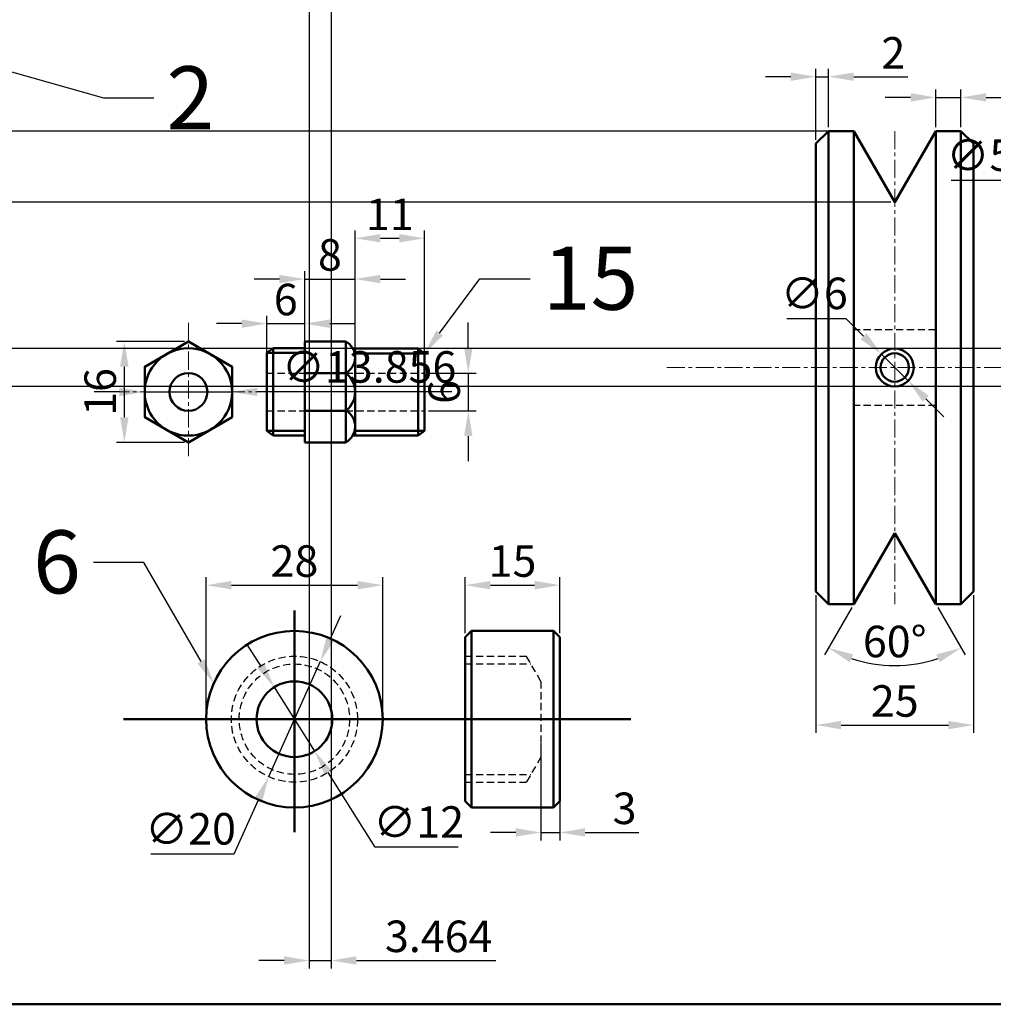
# Model space of a CAD drawing. Units: millimetres. Extents: x 24 to 508, y -182 to 223.
# Tile 3 of 6: x 207 to 361, y -182 to -25. Entities that reach past the tile are written whole.
import ezdxf
from ezdxf import colors
from ezdxf.entities.mleader import LeaderData, LeaderLine
from ezdxf.math import Vec2, Vec3

# ---------------------------------------------------------------- set-up
doc = ezdxf.new("R2010")
doc.units = ezdxf.units.MM
doc.header["$LTSCALE"] = 0.3
doc.linetypes.add('CENTER', pattern=[50.8, 31.75, -6.35, 6.35, -6.35])
doc.linetypes.add('DASHED', pattern=[19.05, 12.7, -6.35])
for name, color, linetype, lineweight in [('M-CNTR', 1, 'CENTER', 18), ('M-DIMS', 2, 'Continuous', 25), ('M-HIDN', 4, 'DASHED', 25), ('M-OUTL', 7, 'Continuous', 50)]:
    doc.layers.add(name, color=color, linetype=linetype, lineweight=lineweight)
doc.styles.get("Standard").update_dxf_attribs({"font": 'arial.ttf'})
doc.dimstyles.new('ISO-25', dxfattribs={"dimtxt": 5, "dimasz": 4, "dimexe": 1.25, "dimexo": 0.625, "dimtad": 1, "dimtoh": 1, "dimdec": 0, "dimtxsty": 'Standard', "dimcen": 2.5, "dimadec": 0, "dimazin": 0, "dimtfac": 1, "dimtdec": 0, "dimtmove": 0, "dimatfit": 3, "dimfxl": 1, "dimarcsym": 0})

# ---------------------------------------------------------------- blocks, each defined once
blk = doc.blocks.new('*D54')
at = {"layer": 'Defpoints', "color": 0, "ltscale": 0.3, "transparency": 16777216}
for p in [(355.8, -37.78), (351.8, -43.11), (355.8, -43.11)]:
    blk.add_point(p, dxfattribs=at)
at = {"layer": 'M-DIMS', "color": 0, "lineweight": -2, "ltscale": 0.3, "transparency": 16777216}
for p, q in [((351.8, -42.48), (351.8, -36.53)), ((355.8, -42.48), (355.8, -36.53)), ((347.8, -37.78), (343.8, -37.78)), ((351.8, -37.78), (355.8, -37.78)), ((359.8, -37.78), (368.51, -37.78))]:
    blk.add_line(p, q, dxfattribs=at)
at = {"layer": 'M-DIMS', "color": 0, "ltscale": 0.3, "transparency": 16777216}
for points in [[(347.8, -37.11), (347.8, -38.44), (351.8, -37.78)], [(359.8, -37.11), (359.8, -38.44), (355.8, -37.78)]]:
    blk.add_solid(points, dxfattribs=at)
at = {"layer": 'M-DIMS', "color": 0, "ltscale": 0.3, "transparency": 16777216, "insert": (366.15, -34.65), "char_height": 5, "attachment_point": 5}
blk.add_mtext('4', dxfattribs=at)
blk = doc.blocks.new('*D55')
at = {"layer": 'Defpoints', "color": 0, "ltscale": 0.3, "transparency": 16777216}
for p in [(332.8, -116.11), (357.8, -116.11), (357.8, -137.3)]:
    blk.add_point(p, dxfattribs=at)
at = {"layer": 'M-DIMS', "color": 0, "lineweight": -2, "ltscale": 0.3, "transparency": 16777216}
for p, q in [((332.8, -116.73), (332.8, -138.55)), ((357.8, -116.73), (357.8, -138.55)), ((336.8, -137.3), (353.8, -137.3))]:
    blk.add_line(p, q, dxfattribs=at)
at = {"layer": 'M-DIMS', "color": 0, "ltscale": 0.3, "transparency": 16777216}
for points in [[(336.8, -136.64), (336.8, -137.97), (332.8, -137.3)], [(353.8, -136.64), (353.8, -137.97), (357.8, -137.3)]]:
    blk.add_solid(points, dxfattribs=at)
at = {"layer": 'M-DIMS', "color": 0, "ltscale": 0.3, "transparency": 16777216, "insert": (345.3, -134.13), "char_height": 5, "attachment_point": 5}
blk.add_mtext('25', dxfattribs=at)
blk = doc.blocks.new('*D56')
at = {"layer": 'Defpoints', "color": 0, "ltscale": 0.3, "transparency": 16777216}
for p in [(345.3, -106.85), (345.3, -106.85), (338.8, -118.11), (351.8, -118.11), (341.65, -127.56)]:
    blk.add_point(p, dxfattribs=at)
at = {"layer": 'M-DIMS', "color": 0, "lineweight": -2, "ltscale": 0.3, "transparency": 16777216}
for p, q in [((338.49, -118.65), (334.16, -126.14)), ((352.11, -118.65), (356.44, -126.14))]:
    blk.add_line(p, q, dxfattribs=at)
blk.add_arc((345.3, -106.85), 21.03, 250.9152, 289.0848, dxfattribs=at)
at = {"layer": 'M-DIMS', "color": 0, "ltscale": 0.3, "transparency": 16777216}
for points in [[(338.15, -127.33), (338.7, -126.11), (334.79, -125.06)], [(351.9, -126.11), (352.45, -127.33), (355.81, -125.06)]]:
    blk.add_solid(points, dxfattribs=at)
at = {"layer": 'M-DIMS', "color": 0, "ltscale": 0.3, "transparency": 16777216, "insert": (345.3, -124.7), "char_height": 5, "attachment_point": 5}
blk.add_mtext('60°', dxfattribs=at)
blk = doc.blocks.new('*D57')
at = {"layer": 'Defpoints', "color": 0, "ltscale": 0.3, "transparency": 16777216}
for p in [(334.8, -34.49), (334.8, -43.11), (332.8, -45.11)]:
    blk.add_point(p, dxfattribs=at)
at = {"layer": 'M-DIMS', "color": 0, "lineweight": -2, "ltscale": 0.3, "transparency": 16777216}
for p, q in [((332.8, -44.48), (332.8, -33.24)), ((334.8, -42.48), (334.8, -33.24)), ((328.8, -34.49), (324.8, -34.49)), ((332.8, -34.49), (334.8, -34.49)), ((338.8, -34.49), (347.36, -34.49))]:
    blk.add_line(p, q, dxfattribs=at)
at = {"layer": 'M-DIMS', "color": 0, "ltscale": 0.3, "transparency": 16777216}
for points in [[(328.8, -33.83), (328.8, -35.16), (332.8, -34.49)], [(338.8, -33.83), (338.8, -35.16), (334.8, -34.49)]]:
    blk.add_solid(points, dxfattribs=at)
at = {"layer": 'M-DIMS', "color": 0, "ltscale": 0.3, "transparency": 16777216, "insert": (345.08, -31.36), "char_height": 5, "attachment_point": 5}
blk.add_mtext('2', dxfattribs=at)
blk = doc.blocks.new('*D58')
at = {"layer": 'Defpoints', "color": 0, "ltscale": 0.3, "transparency": 16777216}
for p in [(251.75, -73.65), (245.75, -84.48), (251.75, -84.48)]:
    blk.add_point(p, dxfattribs=at)
at = {"layer": 'M-DIMS', "color": 0, "lineweight": -2, "ltscale": 0.3, "transparency": 16777216}
for p, q in [((245.75, -83.85), (245.75, -72.4)), ((251.75, -83.85), (251.75, -72.4)), ((241.75, -73.65), (237.75, -73.65)), ((245.75, -73.65), (251.75, -73.65)), ((255.75, -73.65), (259.75, -73.65))]:
    blk.add_line(p, q, dxfattribs=at)
at = {"layer": 'M-DIMS', "color": 0, "ltscale": 0.3, "transparency": 16777216}
for points in [[(241.75, -72.99), (241.75, -74.32), (245.75, -73.65)], [(255.75, -72.99), (255.75, -74.32), (251.75, -73.65)]]:
    blk.add_solid(points, dxfattribs=at)
at = {"layer": 'M-DIMS', "color": 0, "ltscale": 0.3, "transparency": 16777216, "insert": (248.75, -70.47), "char_height": 5, "attachment_point": 5}
blk.add_mtext('6', dxfattribs=at)
blk = doc.blocks.new('*D59')
at = {"layer": 'Defpoints', "color": 0, "ltscale": 0.3, "transparency": 16777216}
for p in [(259.75, -66.58), (251.75, -80.07), (259.75, -80.07)]:
    blk.add_point(p, dxfattribs=at)
at = {"layer": 'M-DIMS', "color": 0, "lineweight": -2, "ltscale": 0.3, "transparency": 16777216}
for p, q in [((251.75, -79.44), (251.75, -65.33)), ((259.75, -79.44), (259.75, -65.33)), ((247.75, -66.58), (243.75, -66.58)), ((251.75, -66.58), (259.75, -66.58)), ((263.75, -66.58), (267.75, -66.58))]:
    blk.add_line(p, q, dxfattribs=at)
at = {"layer": 'M-DIMS', "color": 0, "ltscale": 0.3, "transparency": 16777216}
for points in [[(247.75, -65.91), (247.75, -67.24), (251.75, -66.58)], [(263.75, -65.91), (263.75, -67.24), (259.75, -66.58)]]:
    blk.add_solid(points, dxfattribs=at)
at = {"layer": 'M-DIMS', "color": 0, "ltscale": 0.3, "transparency": 16777216, "insert": (255.75, -63.4), "char_height": 5, "attachment_point": 5}
blk.add_mtext('8', dxfattribs=at)
blk = doc.blocks.new('*D60')
at = {"layer": 'Defpoints', "color": 0, "ltscale": 0.3, "transparency": 16777216}
for p in [(270.75, -60.11), (259.75, -81.48), (270.75, -81.48)]:
    blk.add_point(p, dxfattribs=at)
at = {"layer": 'M-DIMS', "color": 0, "lineweight": -2, "ltscale": 0.3, "transparency": 16777216}
for p, q in [((259.75, -80.85), (259.75, -58.86)), ((270.75, -80.85), (270.75, -58.86)), ((263.75, -60.11), (266.75, -60.11))]:
    blk.add_line(p, q, dxfattribs=at)
at = {"layer": 'M-DIMS', "color": 0, "ltscale": 0.3, "transparency": 16777216}
for points in [[(263.75, -59.44), (263.75, -60.77), (259.75, -60.11)], [(266.75, -59.44), (266.75, -60.77), (270.75, -60.11)]]:
    blk.add_solid(points, dxfattribs=at)
at = {"layer": 'M-DIMS', "color": 0, "ltscale": 0.3, "transparency": 16777216, "insert": (265.25, -56.97), "char_height": 5, "attachment_point": 5}
blk.add_mtext('11', dxfattribs=at)
blk = doc.blocks.new('*D61')
at = {"layer": 'Defpoints', "color": 0, "ltscale": 0.3, "transparency": 16777216}
for p in [(233.32, -76.48), (223.16, -92.48), (233.32, -92.48)]:
    blk.add_point(p, dxfattribs=at)
at = {"layer": 'M-DIMS', "color": 0, "lineweight": -2, "ltscale": 0.3, "transparency": 16777216}
for p, q in [((232.69, -76.48), (221.91, -76.48)), ((223.16, -80.48), (223.16, -88.48)), ((232.69, -92.48), (221.91, -92.48))]:
    blk.add_line(p, q, dxfattribs=at)
at = {"layer": 'M-DIMS', "color": 0, "ltscale": 0.3, "transparency": 16777216}
for points in [[(222.49, -80.48), (223.83, -80.48), (223.16, -76.48)], [(222.49, -88.48), (223.83, -88.48), (223.16, -92.48)]]:
    blk.add_solid(points, dxfattribs=at)
at = {"layer": 'M-DIMS', "color": 0, "ltscale": 0.3, "transparency": 16777216, "insert": (219.98, -84.48), "char_height": 5, "attachment_point": 5, "rotation": 90}
blk.add_mtext('16', dxfattribs=at)
blk = doc.blocks.new('*D62')
at = {"layer": 'Defpoints', "color": 0, "ltscale": 0.3, "transparency": 16777216}
for p in [(270.75, -81.48), (270.75, -87.48), (277.69, -87.48)]:
    blk.add_point(p, dxfattribs=at)
at = {"layer": 'M-DIMS', "color": 0, "lineweight": -2, "ltscale": 0.3, "transparency": 16777216}
for p, q in [((277.69, -77.48), (277.69, -73.48)), ((271.38, -81.48), (278.94, -81.48)), ((277.69, -81.48), (277.69, -87.48)), ((271.38, -87.48), (278.94, -87.48)), ((277.69, -91.48), (277.69, -95.48))]:
    blk.add_line(p, q, dxfattribs=at)
at = {"layer": 'M-DIMS', "color": 0, "ltscale": 0.3, "transparency": 16777216}
for points in [[(277.03, -77.48), (278.36, -77.48), (277.69, -81.48)], [(277.03, -91.48), (278.36, -91.48), (277.69, -87.48)]]:
    blk.add_solid(points, dxfattribs=at)
at = {"layer": 'M-DIMS', "color": 0, "ltscale": 0.3, "transparency": 16777216, "insert": (274.52, -84.48), "char_height": 5, "attachment_point": 5, "rotation": 90}
blk.add_mtext('6', dxfattribs=at)
blk = doc.blocks.new('*D63')
at = {"layer": 'Defpoints', "color": 0, "ltscale": 0.3, "transparency": 16777216}
for p in [(292.21, -115.12), (277.21, -123.37), (292.21, -123.37)]:
    blk.add_point(p, dxfattribs=at)
at = {"layer": 'M-DIMS', "color": 0, "lineweight": -2, "ltscale": 0.3, "transparency": 16777216}
for p, q in [((277.21, -122.74), (277.21, -113.87)), ((292.21, -122.74), (292.21, -113.87)), ((281.21, -115.12), (288.21, -115.12))]:
    blk.add_line(p, q, dxfattribs=at)
at = {"layer": 'M-DIMS', "color": 0, "ltscale": 0.3, "transparency": 16777216}
for points in [[(281.21, -114.45), (281.21, -115.79), (277.21, -115.12)], [(288.21, -114.45), (288.21, -115.79), (292.21, -115.12)]]:
    blk.add_solid(points, dxfattribs=at)
at = {"layer": 'M-DIMS', "color": 0, "ltscale": 0.3, "transparency": 16777216, "insert": (284.71, -111.94), "char_height": 5, "attachment_point": 5}
blk.add_mtext('15', dxfattribs=at)
blk = doc.blocks.new('*D64')
at = {"layer": 'Defpoints', "color": 0, "ltscale": 0.3, "transparency": 16777216}
for p in [(264.13, -115.12), (236.13, -136.37), (264.13, -136.37)]:
    blk.add_point(p, dxfattribs=at)
at = {"layer": 'M-DIMS', "color": 0, "lineweight": -2, "ltscale": 0.3, "transparency": 16777216}
for p, q in [((236.13, -135.74), (236.13, -113.87)), ((264.13, -135.74), (264.13, -113.87)), ((240.13, -115.12), (260.13, -115.12))]:
    blk.add_line(p, q, dxfattribs=at)
at = {"layer": 'M-DIMS', "color": 0, "ltscale": 0.3, "transparency": 16777216}
for points in [[(240.13, -114.45), (240.13, -115.79), (236.13, -115.12)], [(260.13, -114.45), (260.13, -115.79), (264.13, -115.12)]]:
    blk.add_solid(points, dxfattribs=at)
at = {"layer": 'M-DIMS', "color": 0, "ltscale": 0.3, "transparency": 16777216, "insert": (250.13, -111.94), "char_height": 5, "attachment_point": 5}
blk.add_mtext('28', dxfattribs=at)
blk = doc.blocks.new('*D65')
at = {"layer": 'Defpoints', "color": 0, "ltscale": 0.3, "transparency": 16777216}
for p in [(289.21, -139.52), (292.21, -139.52), (292.21, -154.33)]:
    blk.add_point(p, dxfattribs=at)
at = {"layer": 'M-DIMS', "color": 0, "lineweight": -2, "ltscale": 0.3, "transparency": 16777216}
for p, q in [((289.21, -140.15), (289.21, -155.58)), ((292.21, -140.15), (292.21, -155.58)), ((285.21, -154.33), (281.21, -154.33)), ((289.21, -154.33), (292.21, -154.33)), ((296.21, -154.33), (304.74, -154.33))]:
    blk.add_line(p, q, dxfattribs=at)
at = {"layer": 'M-DIMS', "color": 0, "ltscale": 0.3, "transparency": 16777216}
for points in [[(285.21, -153.66), (285.21, -154.99), (289.21, -154.33)], [(296.21, -153.66), (296.21, -154.99), (292.21, -154.33)]]:
    blk.add_solid(points, dxfattribs=at)
at = {"layer": 'M-DIMS', "color": 0, "ltscale": 0.3, "transparency": 16777216, "insert": (302.47, -151.15), "char_height": 5, "attachment_point": 5}
blk.add_mtext('3', dxfattribs=at)
blk = doc.blocks.new('*D66')
at = {"layer": 'Defpoints', "color": 0, "ltscale": 0.3, "transparency": 16777216}
for p in [(246.92, -131.29), (253.33, -141.44)]:
    blk.add_point(p, dxfattribs=at)
at = {"layer": 'M-DIMS', "color": 0, "lineweight": -2, "ltscale": 0.3, "transparency": 16777216}
for p, q in [((244.79, -127.91), (242.65, -124.53)), ((246.92, -131.29), (253.33, -141.44)), ((262.93, -156.64), (255.46, -144.82)), ((276.1, -156.64), (262.93, -156.64))]:
    blk.add_line(p, q, dxfattribs=at)
at = {"layer": 'M-DIMS', "color": 0, "ltscale": 0.3, "transparency": 16777216}
for points in [[(245.35, -127.56), (244.22, -128.27), (246.92, -131.29)], [(256.03, -144.47), (254.9, -145.18), (253.33, -141.44)]]:
    blk.add_solid(points, dxfattribs=at)
at = {"layer": 'M-DIMS', "color": 0, "ltscale": 0.3, "transparency": 16777216, "insert": (269.83, -153.32), "char_height": 5, "attachment_point": 5}
blk.add_mtext('∅12', dxfattribs=at)
blk = doc.blocks.new('*D67')
at = {"layer": 'Defpoints', "color": 0, "ltscale": 0.3, "transparency": 16777216}
for p in [(254.21, -127.24), (246.04, -145.5)]:
    blk.add_point(p, dxfattribs=at)
at = {"layer": 'M-DIMS', "color": 0, "lineweight": -2, "ltscale": 0.3, "transparency": 16777216}
for p, q in [((255.84, -123.59), (257.47, -119.93)), ((254.21, -127.24), (246.04, -145.5)), ((240.58, -157.72), (244.41, -149.15)), ((227.37, -157.72), (240.58, -157.72))]:
    blk.add_line(p, q, dxfattribs=at)
at = {"layer": 'M-DIMS', "color": 0, "ltscale": 0.3, "transparency": 16777216}
for points in [[(255.23, -123.31), (256.45, -123.86), (254.21, -127.24)], [(243.8, -148.88), (245.02, -149.42), (246.04, -145.5)]]:
    blk.add_solid(points, dxfattribs=at)
at = {"layer": 'M-DIMS', "color": 0, "ltscale": 0.3, "transparency": 16777216, "insert": (233.66, -154.4), "char_height": 5, "attachment_point": 5}
blk.add_mtext('∅20', dxfattribs=at)
blk = doc.blocks.new('*D74')
at = {"layer": 'Defpoints', "color": 0, "ltscale": 0.3, "transparency": 16777216}
for p in [(252.48, -2.39), (255.95, -8.39), (255.95, -174.63)]:
    blk.add_point(p, dxfattribs=at)
at = {"layer": 'M-DIMS', "color": 0, "lineweight": -2, "ltscale": 0.3, "transparency": 16777216}
for p, q in [((252.48, -3.01), (252.48, -175.88)), ((255.95, -9.01), (255.95, -175.88)), ((248.48, -174.63), (244.48, -174.63)), ((252.48, -174.63), (255.95, -174.63)), ((259.95, -174.63), (282.05, -174.63))]:
    blk.add_line(p, q, dxfattribs=at)
at = {"layer": 'M-DIMS', "color": 0, "ltscale": 0.3, "transparency": 16777216}
for points in [[(248.48, -173.96), (248.48, -175.3), (252.48, -174.63)], [(259.95, -173.96), (259.95, -175.3), (255.95, -174.63)]]:
    blk.add_solid(points, dxfattribs=at)
at = {"layer": 'M-DIMS', "color": 0, "ltscale": 0.3, "transparency": 16777216, "insert": (273, -171.45), "char_height": 5, "attachment_point": 5}
blk.add_mtext('3.464', dxfattribs=at)
blk = doc.blocks.new('*D76')
at = {"layer": 'Defpoints', "color": 0, "ltscale": 0.3, "transparency": 16777216}
for p in [(411.13, -77.61), (56.57, -83.61), (411.13, -83.61)]:
    blk.add_point(p, dxfattribs=at)
at = {"layer": 'M-DIMS', "color": 0, "lineweight": -2, "ltscale": 0.3, "transparency": 16777216}
for p, q in [((56.57, -73.61), (56.57, -69.61)), ((410.51, -77.61), (55.32, -77.61)), ((56.57, -77.61), (56.57, -83.61)), ((410.51, -83.61), (55.32, -83.61)), ((56.57, -87.61), (56.57, -91.61))]:
    blk.add_line(p, q, dxfattribs=at)
at = {"layer": 'M-DIMS', "color": 0, "ltscale": 0.3, "transparency": 16777216}
for points in [[(55.9, -73.61), (57.24, -73.61), (56.57, -77.61)], [(55.9, -87.61), (57.24, -87.61), (56.57, -83.61)]]:
    blk.add_solid(points, dxfattribs=at)
at = {"layer": 'M-DIMS', "color": 0, "ltscale": 0.3, "transparency": 16777216, "insert": (53.39, -80.61), "char_height": 5, "attachment_point": 5, "rotation": 90}
blk.add_mtext('6', dxfattribs=at)
blk = doc.blocks.new('*D77')
at = {"layer": 'Defpoints', "color": 0, "ltscale": 0.3, "transparency": 16777216}
for p in [(56.57, -43.11), (338.8, -43.11), (345.3, -54.37)]:
    blk.add_point(p, dxfattribs=at)
at = {"layer": 'M-DIMS', "color": 0, "lineweight": -2, "ltscale": 0.3, "transparency": 16777216}
for p, q in [((56.57, -43.11), (56.57, -39.11)), ((56.57, -39.11), (77.49, -39.11)), ((338.18, -43.11), (55.32, -43.11)), ((56.57, -50.37), (56.57, -47.11)), ((344.68, -54.37), (55.32, -54.37))]:
    blk.add_line(p, q, dxfattribs=at)
at = {"layer": 'M-DIMS', "color": 0, "ltscale": 0.3, "transparency": 16777216}
for points in [[(55.9, -47.11), (57.24, -47.11), (56.57, -43.11)], [(55.9, -50.37), (57.24, -50.37), (56.57, -54.37)]]:
    blk.add_solid(points, dxfattribs=at)
at = {"layer": 'M-DIMS', "color": 0, "ltscale": 0.3, "transparency": 16777216, "insert": (67.34, -35.93), "char_height": 5, "attachment_point": 5}
blk.add_mtext('11.258', dxfattribs=at)
blk = doc.blocks.new('*D85')
at = {"layer": 'Defpoints', "color": 0, "ltscale": 0.3, "transparency": 16777216}
for p in [(388.35, -62.05), (425.45, -99.17)]:
    blk.add_point(p, dxfattribs=at)
at = {"layer": 'M-DIMS', "color": 0, "lineweight": -2, "ltscale": 0.3, "transparency": 16777216}
for p, q in [((354.27, -50.91), (377.22, -50.91)), ((377.22, -50.91), (385.52, -59.22)), ((425.45, -99.17), (388.35, -62.05)), ((428.28, -101.99), (431.11, -104.82))]:
    blk.add_line(p, q, dxfattribs=at)
at = {"layer": 'M-DIMS', "color": 0, "ltscale": 0.3, "transparency": 16777216}
for points in [[(385.99, -58.75), (385.05, -59.69), (388.35, -62.05)], [(428.75, -101.52), (427.81, -102.47), (425.45, -99.17)]]:
    blk.add_solid(points, dxfattribs=at)
at = {"layer": 'M-DIMS', "color": 0, "ltscale": 0.3, "transparency": 16777216, "insert": (365.43, -47.59), "char_height": 5, "attachment_point": 5}
blk.add_mtext('∅52.48', dxfattribs=at)
blk = doc.blocks.new('*D86')
at = {"layer": 'Defpoints', "color": 0, "ltscale": 0.3, "transparency": 16777216}
for p in [(343.18, -78.48), (347.42, -82.73)]:
    blk.add_point(p, dxfattribs=at)
at = {"layer": 'M-DIMS', "color": 0, "lineweight": -2, "ltscale": 0.3, "transparency": 16777216}
for p, q in [((328.19, -72.82), (337.53, -72.82)), ((337.53, -72.82), (340.36, -75.65)), ((347.42, -82.73), (343.18, -78.48)), ((350.24, -85.56), (353.07, -88.4))]:
    blk.add_line(p, q, dxfattribs=at)
at = {"layer": 'M-DIMS', "color": 0, "ltscale": 0.3, "transparency": 16777216}
for points in [[(340.83, -75.18), (339.89, -76.12), (343.18, -78.48)], [(350.71, -85.09), (349.77, -86.03), (347.42, -82.73)]]:
    blk.add_solid(points, dxfattribs=at)
at = {"layer": 'M-DIMS', "color": 0, "ltscale": 0.3, "transparency": 16777216, "insert": (332.55, -69.5), "char_height": 5, "attachment_point": 5}
blk.add_mtext('∅6', dxfattribs=at)
blk = doc.blocks.new('*D87')
at = {"layer": 'Defpoints', "color": 0, "ltscale": 0.3, "transparency": 16777216}
for p in [(226.39, -84.48), (240.25, -84.48)]:
    blk.add_point(p, dxfattribs=at)
at = {"layer": 'M-DIMS', "color": 0, "lineweight": -2, "ltscale": 0.3, "transparency": 16777216}
for p, q in [((222.39, -84.48), (218.39, -84.48)), ((226.39, -84.48), (240.25, -84.48)), ((248.25, -84.48), (244.25, -84.48)), ((275.07, -84.48), (248.25, -84.48))]:
    blk.add_line(p, q, dxfattribs=at)
at = {"layer": 'M-DIMS', "color": 0, "ltscale": 0.3, "transparency": 16777216}
for points in [[(222.39, -83.81), (222.39, -85.15), (226.39, -84.48)], [(244.25, -83.81), (244.25, -85.14), (240.25, -84.48)]]:
    blk.add_solid(points, dxfattribs=at)
at = {"layer": 'M-DIMS', "color": 0, "ltscale": 0.3, "transparency": 16777216, "insert": (261.97, -81.16), "char_height": 5, "attachment_point": 5}
blk.add_mtext('∅13.856', dxfattribs=at)

msp = doc.modelspace()

# ---------------------------------------------------------------- linework, layer by layer
at = {"layer": 'M-CNTR', "ltscale": 0.3}
for p, q in [((345.3004, -43.1068), (345.3004, -118.1068)), ((233.3191, -73.5184), (233.3191, -94.8295)), ((467.488, -80.6068), (308.7003, -80.6068)), ((221.1039, -84.4783), (273.9636, -84.4783))]:
    msp.add_line(p, q, dxfattribs=at)
at = {"layer": 'M-HIDN', "ltscale": 0.3}
for p, q in [((351.8004, -74.6068), (338.8004, -74.6068)), ((245.7524, -81.4783), (251.7524, -81.4783)), ((258.2524, -81.4783), (270.7524, -81.4783)), ((351.8004, -86.6068), (338.8004, -86.6068)), ((245.7524, -87.4783), (251.7524, -87.4783)), ((258.2524, -87.4783), (270.7524, -87.4783)), ((277.2109, -126.3679), (286.9015, -126.3679)), ((289.2109, -130.3679), (286.9015, -126.3679)), ((277.2109, -127.6179), (287.6232, -127.6179)), ((289.2109, -130.3679), (289.2109, -142.3679)), ((289.2109, -142.3679), (286.9015, -146.3679)), ((277.2109, -145.1179), (287.6232, -145.1179)), ((277.2109, -146.3679), (286.9015, -146.3679))]:
    msp.add_line(p, q, dxfattribs=at)
for radius in [10, 8.75]:
    msp.add_circle((250.1252, -136.3679), radius, dxfattribs=at)
at = {"layer": 'M-OUTL', "ltscale": 0.3}
for p, q in [((332.8004, -45.1068), (334.8004, -43.1068)), ((334.8004, -43.1068), (334.8004, -118.1068)), ((338.8004, -43.1068), (334.8004, -43.1068)), ((338.8004, -43.1068), (338.8004, -118.1068)), ((338.8004, -43.1068), (345.3004, -54.3651)), ((351.8004, -43.1068), (345.3004, -54.3651)), ((355.8004, -43.1068), (351.8004, -43.1068)), ((351.8004, -118.1068), (351.8004, -43.1068)), ((355.8004, -118.1068), (355.8004, -43.1068)), ((357.8004, -45.1068), (355.8004, -43.1068)), ((332.8004, -45.1068), (332.8004, -116.1068)), ((357.8004, -116.1068), (357.8004, -45.1068)), ((251.7524, -76.4783), (258.2524, -76.4783)), ((251.7524, -77.5501), (251.7524, -76.4783)), ((258.2524, -76.4783), (258.2524, -92.4783)), ((245.7524, -78.3001), (246.7524, -77.5501)), ((246.7524, -77.5501), (251.7524, -77.5501)), ((246.7524, -77.5501), (246.7524, -91.4065)), ((251.7524, -77.5501), (251.7524, -91.4065)), ((259.4369, -77.6143), (269.7524, -77.6143)), ((259.7524, -77.6143), (259.7524, -91.4065)), ((269.7524, -77.6143), (269.7524, -91.4065)), ((269.7524, -77.6143), (270.7524, -78.3643)), ((245.7524, -78.3001), (245.7524, -90.6565)), ((245.7524, -78.3001), (251.7524, -78.3001)), ((259.6851, -78.3643), (270.7524, -78.3643)), ((270.7524, -78.3643), (270.7524, -90.6565)), ((251.7524, -81.4783), (258.2524, -81.4783)), ((251.7524, -87.4783), (258.3793, -87.4783)), ((251.7524, -90.6565), (245.7524, -90.6565)), ((245.7524, -90.6565), (246.7524, -91.4065)), ((251.7524, -91.4065), (246.7524, -91.4065)), ((251.7524, -91.4065), (251.7524, -92.4783)), ((269.7524, -91.4065), (259.3905, -91.4065)), ((270.7524, -90.6565), (259.6628, -90.6565)), ((270.7524, -90.6565), (269.7524, -91.4065)), ((251.7524, -92.4783), (258.2524, -92.4783)), ((338.8004, -118.1068), (345.3004, -106.8485)), ((351.8004, -118.1068), (345.3004, -106.8485)), ((332.8004, -116.1068), (334.8004, -118.1068)), ((357.8004, -116.1068), (355.8004, -118.1068)), ((334.8004, -118.1068), (338.8004, -118.1068)), ((351.8004, -118.1068), (355.8004, -118.1068)), ((250.1252, -119.1606), (250.1252, -154.2807)), ((278.2109, -122.3679), (277.2109, -123.3679)), ((278.2109, -122.3679), (291.2109, -122.3679)), ((278.2109, -150.3679), (278.2109, -122.3679)), ((291.2109, -122.3679), (291.2109, -150.3679)), ((292.2109, -123.3679), (291.2109, -122.3679)), ((277.2109, -149.3679), (277.2109, -123.3679)), ((292.2109, -123.3679), (292.2109, -149.3679)), ((303.4354, -136.3679), (223.0395, -136.3679)), ((277.2109, -149.3679), (278.2109, -150.3679)), ((292.2109, -149.3679), (291.2109, -150.3679)), ((291.2109, -150.3679), (278.2109, -150.3679))]:
    msp.add_line(p, q, dxfattribs=at)
for points in [[(23.7253, 222.7463), (508.4225, 222.7463), (508.4225, -181.5799), (23.7253, -181.5799)], [(233.3191, -76.4783), (226.3909, -80.4783), (226.3909, -88.4783), (233.3191, -92.4783), (240.2473, -88.4783), (240.2473, -80.4783)]]:
    msp.add_lwpolyline(points, close=True, dxfattribs=at)
for centre, radius in [((233.3191, -84.4783), 6.9282), ((345.3004, -80.6068), 3), ((345.3004, -80.6068), 2.25), ((233.3191, -84.4783), 3), ((250.1252, -136.3679), 14), ((250.1252, -136.3679), 6)]:
    msp.add_circle(centre, radius, dxfattribs=at)
for centre, radius, start, end in [((256.919, -78.9783), 2.8333, 298.072487, 61.927513), ((256.0024, -84.4783), 3.75, 306.869898, 53.130102), ((256.8573, -89.9413), 2.8953, 298.806556, 59.927872)]:
    msp.add_arc(centre, radius, start, end, dxfattribs=at)

# ---------------------------------------------------------------- dimensions: what is measured, and where the dimension line sits
at = {"layer": 'M-DIMS', "ltscale": 0.3}
for base, p1, p2, override, picture, middle in [((255.9466, -174.6307), (252.4824, -2.3853), (255.9466, -8.3853), {"dimdec": 3, "dimlfac": 1, "dimrnd": 0, "dimzin": 0, "dimdsep": 46, "dimlunit": 2}, '*D74', (272.9958, -171.4511)), ((334.8004, -34.4917), (332.8004, -45.1068), (334.8004, -43.1068), {"dimclrd": 0, "dimclre": 0, "dimclrt": 0}, '*D57', (345.0813, -31.3565)), ((355.8004, -37.7754), (351.8004, -43.1068), (355.8004, -43.1068), {"dimclrd": 0, "dimclre": 0, "dimclrt": 0}, '*D54', (366.1546, -34.6504)), ((270.7524, -60.108), (259.7524, -81.4783), (270.7524, -81.4783), {"dimclrd": 0, "dimclre": 0, "dimclrt": 0}, '*D60', (265.2524, -56.9728)), ((259.7524, -66.5763), (251.7524, -80.066), (259.7524, -80.066), {"dimclrd": 0, "dimclre": 0, "dimclrt": 0}, '*D59', (255.7524, -63.3984)), ((251.7524, -73.6522), (245.7524, -84.4783), (251.7524, -84.4783), {"dimclrd": 0, "dimclre": 0, "dimclrt": 0}, '*D58', (248.7524, -70.4743)), ((264.1252, -115.1185), (236.1252, -136.3679), (264.1252, -136.3679), {"dimclrd": 0, "dimclre": 0, "dimclrt": 0}, '*D64', (250.1252, -111.9407)), ((292.2109, -115.1185), (277.2109, -123.3679), (292.2109, -123.3679), {"dimclrd": 0, "dimclre": 0, "dimclrt": 0}, '*D63', (284.7109, -111.9407)), ((357.8004, -137.3047), (332.8004, -116.1068), (357.8004, -116.1068), {"dimclrd": 0, "dimclre": 0, "dimclrt": 0}, '*D55', (345.3004, -134.1269)), ((292.2109, -154.3272), (289.2109, -139.5205), (292.2109, -139.5205), {"dimclrd": 0, "dimclre": 0, "dimclrt": 0}, '*D65', (302.473, -151.1476))]:
    dim = msp.add_linear_dim(base=base, p1=p1, p2=p2, dimstyle='ISO-25', override=override, dxfattribs=at)
    dim.commit()
    dim.dimension.update_dxf_attribs({"geometry": picture, "text_midpoint": middle})
for base, p1, p2, override, picture, middle in [((56.5704, -43.1068), (345.3004, -54.3651), (338.8004, -43.1068), {"dimdec": 3, "dimlfac": 1, "dimrnd": 0, "dimzin": 0, "dimdsep": 46, "dimlunit": 2}, '*D77', (67.3438, -35.9289)), ((56.5704, -83.6068), (411.1321, -77.6068), (411.1321, -83.6068), {"dimdec": 0, "dimlfac": 1, "dimrnd": 0, "dimzin": 0, "dimdsep": 46, "dimlunit": 2}, '*D76', (53.3925, -80.6068)), ((277.6937, -87.4783), (270.7524, -81.4783), (270.7524, -87.4783), {"dimclrd": 0, "dimclre": 0, "dimclrt": 0}, '*D62', (274.5159, -84.4783)), ((223.1587, -92.4783), (233.3191, -76.4783), (233.3191, -92.4783), {"dimclrd": 0, "dimclre": 0, "dimclrt": 0}, '*D61', (219.9808, -84.4783))]:
    dim = msp.add_linear_dim(base=base, p1=p1, p2=p2, angle=90, dimstyle='ISO-25', override=override, dxfattribs=at)
    dim.commit()
    dim.dimension.update_dxf_attribs({"geometry": picture, "text_midpoint": middle})
for p1, p2, override, picture, middle in [((425.453, -99.1656), (388.348, -62.048), {"dimdec": 2, "dimlfac": 1, "dimrnd": 0, "dimzin": 0, "dimdsep": 46, "dimlunit": 2}, '*D85', (365.4301, -50.9127)), ((347.4185, -82.7313), (343.1823, -78.4823), {"dimdec": 0, "dimlfac": 1, "dimrnd": 0, "dimzin": 0, "dimdsep": 46, "dimlunit": 2}, '*D86', (332.552, -72.8168)), ((226.3909, -84.4786), (240.2473, -84.478), {"dimdec": 3, "dimlfac": 1, "dimrnd": 0, "dimzin": 0, "dimdsep": 46, "dimlunit": 2}, '*D87', (248.2473, -84.4777)), ((246.9218, -131.2946), (253.3286, -141.4412), {"dimclrd": 0, "dimclre": 0, "dimclrt": 0}, '*D66', (269.8258, -156.6398))]:
    dim = msp.add_diameter_dim_2p(p1=p1, p2=p2, dimstyle='ISO-25', override=override, dxfattribs=at)
    dim.commit()
    dim.dimension.update_dxf_attribs({"geometry": picture, "text_midpoint": middle, "dimtype": 163})
dim = msp.add_angular_dim_2l(base=(341.6489, -127.5574), line1=((351.8004, -118.1068), (345.3004, -106.8485)), line2=((338.8004, -118.1068), (345.3004, -106.8485)), dimstyle='ISO-25', override={"dimclrd": 0, "dimclre": 0, "dimclrt": 0}, dxfattribs=at)
dim.commit()
dim.dimension.update_dxf_attribs({"geometry": '*D56', "text_midpoint": (345.3004, -124.699)})
dim = msp.add_diameter_dim_2p(p1=(254.206, -127.2384), p2=(246.0444, -145.4973), dimstyle='ISO-25', override={"dimclrd": 0, "dimclre": 0, "dimclrt": 0}, dxfattribs=at)
dim.commit()
dim.dimension.update_dxf_attribs({"geometry": '*D67', "text_midpoint": (233.6644, -154.3998)})

# ---------------------------------------------------------------- leaders
ml = msp.add_multileader_mtext('Standard', dxfattribs=at)
ml.set_content('2', color=256)
ml.set_leader_properties()
ml.build(insert=Vec2(0, 0))
ctx = ml.context
ctx.base_point, ctx.char_height, ctx.plane_origin = Vec3(227.8339, -37.8459), 10, Vec3(188.3582, -28.9708)
notes = []
notes.append((ctx, [(0, (1, 1, 0), (219.8339, -37.8459), (1, 0), 8, [(0, [(188.3582, -28.9708)], 0, [])])]))
ctx.mtext.insert, ctx.mtext.flow_direction = Vec3(229.8339, -32.8459), 5
ml = msp.add_multileader_mtext('Standard', dxfattribs=at)
ml.set_content('15', color=256)
ml.set_leader_properties()
ml.build(insert=Vec2(0, 0))
ctx = ml.context
ctx.base_point, ctx.char_height, ctx.plane_origin = Vec3(287.5022, -66.5317), 10, Vec3(270.7524, -78.3643)
notes.append((ctx, [(0, (1, 1, 0), (279.5022, -66.5317), (1, 0), 8, [(0, [(270.7524, -78.3643)], 0, [])])]))
ctx.mtext.insert, ctx.mtext.flow_direction = Vec3(289.5022, -61.4464), 5
ml = msp.add_multileader_mtext('Standard', dxfattribs=at)
ml.set_content('6', color=256)
ml.set_leader_properties()
ml.build(insert=Vec2(0, 0))
ctx = ml.context
ctx.base_point, ctx.char_height, ctx.plane_origin = Vec3(207.6595, -111.5112), 10, Vec3(237.3314, -130.683)
ctx.text_align_type = 2
notes.append((ctx, [(0, (1, 1, 0), (226.2625, -111.5112), (-1, 0), 8, [(0, [(237.3314, -130.683)], 0, [])])]))
ctx.mtext.insert, ctx.mtext.alignment, ctx.mtext.flow_direction = Vec3(216.2625, -106.4259), 3, 5
for ctx, leaders in notes:
    for number, flags, end, landing, length, lines in leaders:
        leader = LeaderData()
        leader.index, (leader.has_last_leader_line, leader.has_dogleg_vector, leader.attachment_direction) = number, flags
        leader.last_leader_point, leader.dogleg_vector, leader.dogleg_length = Vec3(end), Vec3(landing), length
        for number, points, colour, breaks in lines:
            line = LeaderLine()
            line.index, line.vertices, line.color, line.breaks = number, Vec3.list(points), colors.encode_raw_color(colour), breaks
            leader.lines.append(line)
        ctx.leaders.append(leader)

doc.saveas('drawing.dxf')
